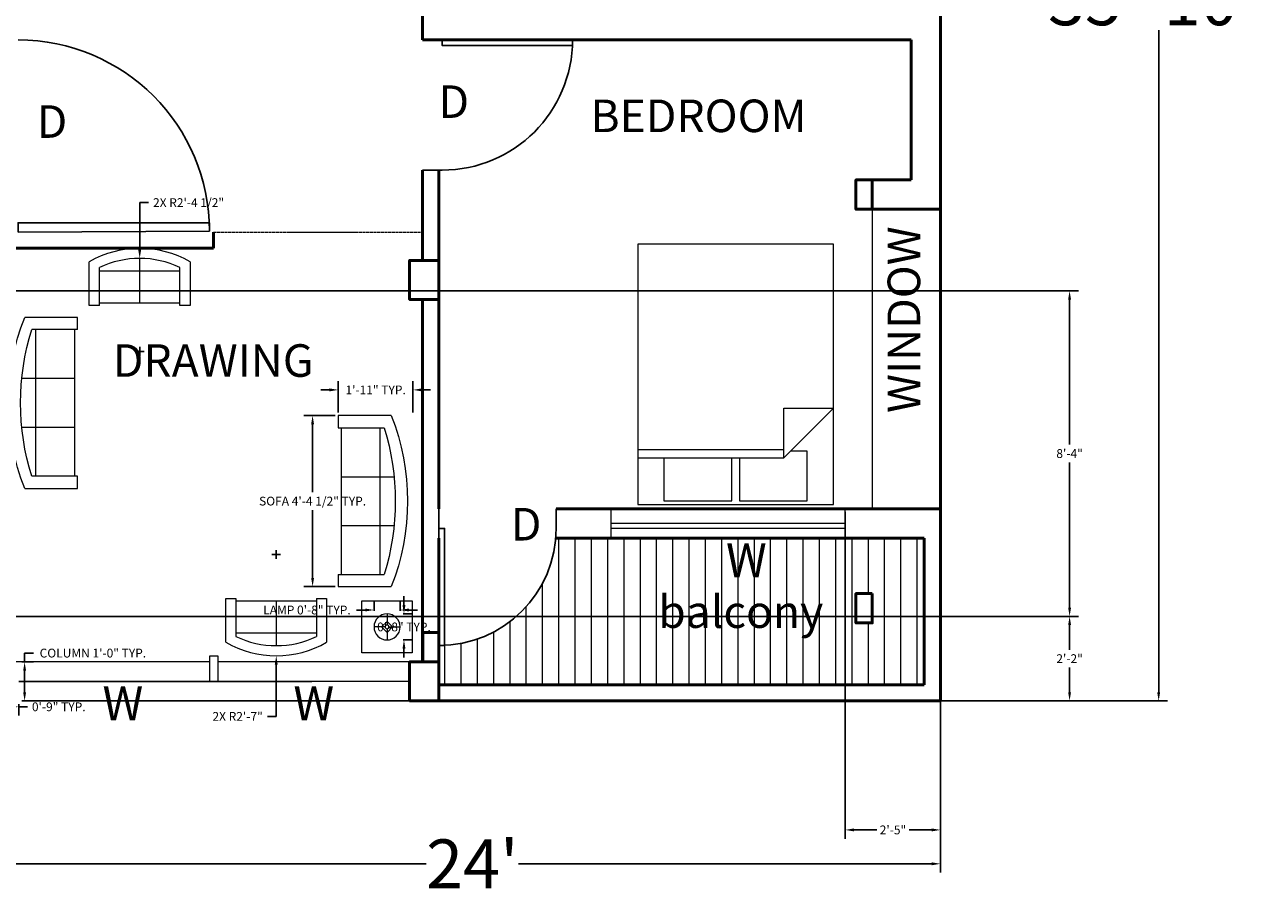
# Model space of a CAD drawing. Units: inches. Extents: x -15 to 796, y 111 to 651.
# Tile 5 of 6: x 416 to 796, y 111 to 376. Entities that reach past the tile are written whole.
import ezdxf

# ---------------------------------------------------------------- set-up
doc = ezdxf.new("R2010")
doc.units = ezdxf.units.IN
doc.header["$MEASUREMENT"] = 0
doc.linetypes.add('DASHED2', pattern=[0.375, 0.25, -0.125])
doc.layers.get('0').update_dxf_attribs({"color": 1})
for name, color, linetype, lineweight in [('A-ANNO-DIMS', 2, 'Continuous', 18), ('A-ANNO-TEXT', 7, 'Continuous', 18), ('A-AREA-IDEN', 7, 'Continuous', 25), ('A-COLS', 1, 'Continuous', 50), ('A-DOOR', 3, 'Continuous', 25), ('A-FLOR-PATT', 18, 'Continuous', 13), ('A-FURN', 8, 'Continuous', 18), ('A-GLAZ', 4, 'Continuous', 18), ('A-WALL', 7, 'Continuous', 50), ('A-WALL-OVHD', 7, 'DASHED2', 18)]:
    doc.layers.add(name, color=color, linetype=linetype, lineweight=lineweight)
doc.styles.get("Standard").update_dxf_attribs({"font": 'arial.ttf'})
doc.dimstyles.get("Standard").update_dxf_attribs({"dimscale": 15, "dimtxt": 0.18, "dimasz": 0.18, "dimexe": 0.18, "dimexo": 0.0625, "dimgap": 0.09, "dimtad": 0, "dimtih": 1, "dimtoh": 1, "dimdec": 0, "dimzin": 0, "dimdsep": 46, "dimlunit": 3, "dimtxsty": 'Standard', "dimcen": 0.09, "dimadec": 0, "dimazin": 0, "dimtfac": 1, "dimtdec": 0, "dimtofl": 0, "dimtmove": 0, "dimatfit": 3, "dimfxl": 1, "dimtolj": 1, "dimtzin": 0, "dimarcsym": 0})

# ---------------------------------------------------------------- blocks, each defined once
blk = doc.blocks.new('*U2')
for p, q in [((-36, 0), (-36, 6)), ((0, 0), (0, 6))]:
    blk.add_line(p, q)
blk.add_lwpolyline([(0, 0), (0, -36), (-1.75, -36), (-1.75, 0)], close=True)
blk.add_arc((0, 0), 36, 180, 270)
blk = doc.blocks.new('Bed - Queen')
for p, q in [((0, -80.00003), (0, 0)), ((0, 0), (59.99999, 0)), ((59.99999, 0), (59.99999, -80.00003)), ((7.99999, -1.2), (28.79998, -1.2)), ((7.99999, -14.4), (7.99999, -1.2)), ((28.79998, -1.2), (28.79998, -14.4)), ((31.19999, -1.2), (51.99999, -1.2)), ((31.19999, -14.4), (31.19999, -1.2)), ((51.99999, -1.2), (51.99999, -16.4)), ((0, -14.4), (44.8, -14.4)), ((59.99999, -29.6), (44.8, -14.4)), ((44.8, -14.4), (44.8, -29.6)), ((44.8, -16.8), (0, -16.8)), ((51.99999, -16.4), (46.79936, -16.4)), ((44.8, -29.6), (59.99999, -29.6)), ((59.99999, -80.00003), (0, -80.00003))]:
    blk.add_line(p, q)
blk = doc.blocks.new('*U4')
for p, q in [((0, 0), (0, -6)), ((-40, 0), (-40, -6))]:
    blk.add_line(p, q)
blk.add_lwpolyline([(0, 0), (0, 40), (-1.75, 40), (-1.75, 0)], close=True)
blk.add_arc((0, 0), 40, 90, 180)
blk = doc.blocks.new('Sofa - Roundback Loveseat 5 ft.')
for p, q in [((0, -32.44198), (0, -5.99998)), ((-24, -33.99998), (-24, -11.46958)), ((-23.9998, -13.38178), (23.99986, -13.38178)), ((24.00004, -33.99998), (24.00004, -11.46958)), ((-24, -32.44198), (24.00004, -32.44198))]:
    blk.add_line(p, q)
for points in [[(-24, -33.99998), (-30, -33.99998), (-30, -7.99998)], [(30.00004, -7.99998), (30.00004, -33.99998), (24.00004, -33.99998)]]:
    blk.add_lwpolyline(points)
for centre, radius, start, end in [((0, -60.24998), 60.24998, 60.13715, 119.8628), ((0, -61.38438), 55.38444, 64.32083, 115.6792)]:
    blk.add_arc(centre, radius, start, end)
blk = doc.blocks.new('Lamp - Table')
for p, q in [((0, 7), (0, 1)), ((-1, 0), (-7, 0)), ((0, 3), (-3, 0)), ((-3, 0), (0, -3)), ((3, 0), (0, 3)), ((0, -3), (3, 0)), ((1, 0), (7, 0)), ((0, -1), (0, -7))]:
    blk.add_line(p, q)
for radius in [7, 1]:
    blk.add_circle((0, 0), radius)
blk = doc.blocks.new('Sofa - Roundback 7 ft.')
for p, q in [((-36.000027, -34), (-36.000027, -11.4696)), ((-12.00002, -32.4421), (-12.00003, -6.5971)), ((11.99997, -32.4421), (11.99998, -6.5971)), ((35.99998, -34), (35.99998, -11.4696)), ((-35.999844, -13.3819), (35.9998, -13.3819)), ((-36.000027, -32.4421), (35.99998, -32.4421))]:
    blk.add_line(p, q)
for points in [[(-36.000027, -34), (-42.000027, -34), (-42.000027, -8)], [(41.99998, -8), (41.99998, -34), (35.99998, -34)]]:
    blk.add_lwpolyline(points)
for centre, radius, start, end in [((0, -114.25), 114.25, 68.43141, 111.5686), ((-0.00001, -127.1968), 121.1968, 72.72033, 107.2797)]:
    blk.add_arc(centre, radius, start, end)
blk = doc.blocks.new('*D17')
at = {"layer": 'A-ANNO-DIMS', "color": 0, "lineweight": -2, "transparency": 16777216}
for p, q in [((698.12, 598.13), (766.83, 598.13)), ((764.13, 595.43), (764.13, 392.14)), ((764.13, 170.83), (764.13, 374.11)), ((698.12, 168.13), (766.83, 168.13))]:
    blk.add_line(p, q, dxfattribs=at)
at = {"layer": 'A-ANNO-DIMS', "color": 0, "transparency": 16777216}
for points in [[(763.68, 595.43), (764.58, 595.43), (764.13, 598.13)], [(763.68, 170.83), (764.58, 170.83), (764.13, 168.13)]]:
    blk.add_solid(points, dxfattribs=at)
at = {"layer": 'Defpoints', "color": 0, "transparency": 16777216}
for p in [(697.18, 598.13), (697.18, 168.13), (764.13, 168.13)]:
    blk.add_point(p, dxfattribs=at)
at = {"layer": 'A-ANNO-DIMS', "color": 0, "transparency": 16777216, "insert": (764.13, 383.13), "char_height": 2.7, "attachment_point": 5}
blk.add_mtext('\\A1;{\\H5.55556x;35\'-10"}', dxfattribs=at)
blk = doc.blocks.new('*D18')
at = {"layer": 'A-ANNO-DIMS', "color": 0, "lineweight": -2, "transparency": 16777216}
for p, q in [((409.68, 179.19), (409.68, 115.42)), ((697.18, 179.19), (697.18, 115.42)), ((412.38, 118.12), (539.23, 118.12)), ((694.48, 118.12), (567.64, 118.12))]:
    blk.add_line(p, q, dxfattribs=at)
at = {"layer": 'A-ANNO-DIMS', "color": 0, "transparency": 16777216}
for points in [[(412.38, 118.57), (412.38, 117.67), (409.68, 118.12)], [(694.48, 118.57), (694.48, 117.67), (697.18, 118.12)]]:
    blk.add_solid(points, dxfattribs=at)
at = {"layer": 'Defpoints', "color": 0, "transparency": 16777216}
for p in [(409.68, 180.13), (697.18, 180.13), (697.18, 118.12)]:
    blk.add_point(p, dxfattribs=at)
at = {"layer": 'A-ANNO-DIMS', "color": 0, "transparency": 16777216, "insert": (553.43, 118.12), "char_height": 2.7, "attachment_point": 5}
blk.add_mtext("\\A1;{\\H5.55556x;24'}", dxfattribs=at)
blk = doc.blocks.new('DOOR-ENTRY-59IN')
blk.add_lwpolyline([(0, -0.29), (-58.71, 0), (-58.71, 2.57), (0, 2.57)], close=True)
blk.add_arc((0, 0), 58.71, 90, 180)
blk = doc.blocks.new('WIN-BEDROOM-72IN')
for p, q in [((0, 4.5), (72, 4.5)), ((0, 2.96), (72, 2.96))]:
    blk.add_line(p, q)
blk.add_lwpolyline([(0, 9), (72, 9), (72, 0), (0, 0)], close=True)
blk = doc.blocks.new('WIN-LIVING-PAIRED')
for p, q in [((62.78, 7.78), (65.45, 7.78)), ((62.78, 0), (62.78, 7.78)), ((65.45, 7.78), (65.45, 0)), ((0, 6), (62.78, 6)), ((65.45, 6), (128.5, 6)), ((4, 0), (124, 0)), ((65.45, 0), (62.78, 0))]:
    blk.add_line(p, q)
blk = doc.blocks.new('COL-9X12')
blk.add_lwpolyline([(9, 0), (0, 0), (0, 12), (9, 12)], close=True)
blk = doc.blocks.new('PIER-5X9')
blk.add_lwpolyline([(0, 9), (5, 9), (5, 0), (0, 0)], close=True)
blk = doc.blocks.new('TABLE-LAMP-STAND')
blk.add_lwpolyline([(0, 0), (15.51, 0), (15.51, 15.93), (0, 15.93)], close=True)
blk = doc.blocks.new('*D35')
at = {"layer": 'A-ANNO-DIMS', "color": 0, "lineweight": -2, "transparency": 16777216}
for p, q in [((415.98, 180.13), (415.98, 182.83)), ((415.98, 182.83), (418.68, 182.83)), ((415.12, 180.13), (418.68, 180.13)), ((415.98, 170.83), (415.98, 177.43)), ((415.12, 168.13), (418.68, 168.13))]:
    blk.add_line(p, q, dxfattribs=at)
at = {"layer": 'A-ANNO-DIMS', "color": 0, "transparency": 16777216}
for points in [[(415.53, 177.43), (416.43, 177.43), (415.98, 180.13)], [(415.53, 170.83), (416.43, 170.83), (415.98, 168.13)]]:
    blk.add_solid(points, dxfattribs=at)
at = {"layer": 'Defpoints', "color": 0, "transparency": 16777216}
for p in [(414.18, 180.13), (415.98, 180.13), (414.18, 168.13)]:
    blk.add_point(p, dxfattribs=at)
at = {"layer": 'A-ANNO-DIMS', "color": 0, "transparency": 16777216, "insert": (436.94, 182.83), "char_height": 2.7, "attachment_point": 5}
blk.add_mtext('\\A1;COLUMN 1\'-0" TYP.', dxfattribs=at)
blk = doc.blocks.new('*D36')
at = {"layer": 'A-ANNO-DIMS', "color": 0, "lineweight": -2, "transparency": 16777216}
for p, q in [((405.18, 167.19), (405.18, 163.63)), ((407.88, 166.33), (411.48, 166.33)), ((414.18, 167.19), (414.18, 163.63)), ((414.18, 166.33), (416.88, 166.33))]:
    blk.add_line(p, q, dxfattribs=at)
at = {"layer": 'A-ANNO-DIMS', "color": 0, "transparency": 16777216}
for points in [[(407.88, 166.78), (407.88, 165.88), (405.18, 166.33)], [(411.48, 166.78), (411.48, 165.88), (414.18, 166.33)]]:
    blk.add_solid(points, dxfattribs=at)
at = {"layer": 'Defpoints', "color": 0, "transparency": 16777216}
for p in [(405.18, 168.13), (414.18, 168.13), (414.18, 166.33)]:
    blk.add_point(p, dxfattribs=at)
at = {"layer": 'A-ANNO-DIMS', "color": 0, "transparency": 16777216, "insert": (426.46, 166.33), "char_height": 2.7, "attachment_point": 5}
blk.add_mtext('\\A1;0\'-9" TYP.', dxfattribs=at)
blk = doc.blocks.new('*D43')
at = {"layer": 'A-ANNO-DIMS', "color": 0, "lineweight": -2, "transparency": 16777216}
for p, q in [((511.33, 255.77), (501.69, 255.77)), ((504.39, 253.07), (504.39, 232.24)), ((504.39, 205.93), (504.39, 226.75)), ((511.33, 203.23), (501.69, 203.23))]:
    blk.add_line(p, q, dxfattribs=at)
at = {"layer": 'A-ANNO-DIMS', "color": 0, "transparency": 16777216}
for points in [[(503.94, 253.07), (504.84, 253.07), (504.39, 255.77)], [(503.94, 205.93), (504.84, 205.93), (504.39, 203.23)]]:
    blk.add_solid(points, dxfattribs=at)
at = {"layer": 'Defpoints', "color": 0, "transparency": 16777216}
for p in [(504.39, 255.77), (512.27, 255.77), (512.27, 203.23)]:
    blk.add_point(p, dxfattribs=at)
at = {"layer": 'A-ANNO-DIMS', "color": 0, "transparency": 16777216, "insert": (504.39, 229.5), "char_height": 2.7, "attachment_point": 5}
blk.add_mtext('\\A1;SOFA 4\'-4 1/2" TYP.', dxfattribs=at)
blk = doc.blocks.new('*D44')
at = {"layer": 'A-ANNO-DIMS', "color": 0, "lineweight": -2, "transparency": 16777216}
for p, q in [((512.27, 256.71), (512.27, 266.35)), ((535.21, 256.71), (535.21, 266.35)), ((509.57, 263.65), (506.87, 263.65)), ((537.91, 263.65), (540.61, 263.65))]:
    blk.add_line(p, q, dxfattribs=at)
at = {"layer": 'A-ANNO-DIMS', "color": 0, "transparency": 16777216}
for points in [[(509.57, 264.1), (509.57, 263.2), (512.27, 263.65)], [(537.91, 264.1), (537.91, 263.2), (535.21, 263.65)]]:
    blk.add_solid(points, dxfattribs=at)
at = {"layer": 'Defpoints', "color": 0, "transparency": 16777216}
for p in [(535.21, 263.65), (512.27, 255.77), (535.21, 255.77)]:
    blk.add_point(p, dxfattribs=at)
at = {"layer": 'A-ANNO-DIMS', "color": 0, "transparency": 16777216, "insert": (523.74, 263.65), "char_height": 2.7, "attachment_point": 5}
blk.add_mtext('\\A1;1\'-11" TYP.', dxfattribs=at)
blk = doc.blocks.new('*D49')
at = {"layer": 'A-ANNO-DIMS', "color": 0, "lineweight": -2, "transparency": 16777216}
for p, q in [((523.24, 195.8), (523.24, 198.76)), ((531.24, 195.8), (531.24, 198.76)), ((520.54, 196.06), (517.84, 196.06)), ((533.94, 196.06), (536.64, 196.06))]:
    blk.add_line(p, q, dxfattribs=at)
at = {"layer": 'A-ANNO-DIMS', "color": 0, "transparency": 16777216}
for points in [[(520.54, 196.51), (520.54, 195.61), (523.24, 196.06)], [(533.94, 196.51), (533.94, 195.61), (531.24, 196.06)]]:
    blk.add_solid(points, dxfattribs=at)
at = {"layer": 'Defpoints', "color": 0, "transparency": 16777216}
for p in [(523.24, 196.06), (523.24, 194.86), (531.24, 194.86)]:
    blk.add_point(p, dxfattribs=at)
at = {"layer": 'A-ANNO-DIMS', "color": 0, "transparency": 16777216, "insert": (502.66, 196.06), "char_height": 2.7, "attachment_point": 5}
blk.add_mtext('\\A1;LAMP 0\'-8" TYP.', dxfattribs=at)
blk = doc.blocks.new('*D50')
at = {"layer": 'A-ANNO-DIMS', "color": 0, "lineweight": -2, "transparency": 16777216}
for p, q in [((532.44, 197.56), (532.44, 200.26)), ((532.18, 194.86), (535.14, 194.86)), ((532.18, 186.86), (535.14, 186.86)), ((532.44, 184.16), (532.44, 181.46))]:
    blk.add_line(p, q, dxfattribs=at)
at = {"layer": 'A-ANNO-DIMS', "color": 0, "transparency": 16777216}
for points in [[(531.99, 197.56), (532.89, 197.56), (532.44, 194.86)], [(531.99, 184.16), (532.89, 184.16), (532.44, 186.86)]]:
    blk.add_solid(points, dxfattribs=at)
at = {"layer": 'Defpoints', "color": 0, "transparency": 16777216}
for p in [(531.24, 194.86), (532.44, 194.86), (531.24, 186.86)]:
    blk.add_point(p, dxfattribs=at)
at = {"layer": 'A-ANNO-DIMS', "color": 0, "transparency": 16777216, "insert": (532.44, 190.86), "char_height": 2.7, "attachment_point": 5}
blk.add_mtext('\\A1;0\'-8" TYP.', dxfattribs=at)
blk = doc.blocks.new('*D68')
at = {"layer": 'A-ANNO-DIMS', "color": 0, "lineweight": -2, "transparency": 16777216}
for p, q in [((366.85, 294.11), (739.48, 294.11)), ((736.78, 291.41), (736.78, 246.84)), ((736.78, 196.81), (736.78, 241.38)), ((366.85, 194.11), (739.48, 194.11))]:
    blk.add_line(p, q, dxfattribs=at)
at = {"layer": 'A-ANNO-DIMS', "color": 0, "transparency": 16777216}
for points in [[(736.33, 291.41), (737.23, 291.41), (736.78, 294.11)], [(736.33, 196.81), (737.23, 196.81), (736.78, 194.11)]]:
    blk.add_solid(points, dxfattribs=at)
at = {"layer": 'Defpoints', "color": 0, "transparency": 16777216}
for p in [(365.91, 294.11), (736.78, 294.11), (365.91, 194.11)]:
    blk.add_point(p, dxfattribs=at)
at = {"layer": 'A-ANNO-DIMS', "color": 0, "transparency": 16777216, "insert": (736.78, 244.11), "char_height": 2.7, "attachment_point": 5}
blk.add_mtext('\\A1;8\'-4"', dxfattribs=at)
blk = doc.blocks.new('*D77')
at = {"layer": 'A-ANNO-DIMS', "color": 0, "lineweight": -2, "transparency": 16777216}
for p, q in [((667.93, 226.19), (667.93, 125.83)), ((697.18, 226.19), (697.18, 125.83)), ((670.63, 128.53), (677.6, 128.53)), ((694.48, 128.53), (687.52, 128.53))]:
    blk.add_line(p, q, dxfattribs=at)
at = {"layer": 'A-ANNO-DIMS', "color": 0, "transparency": 16777216}
for points in [[(670.63, 128.98), (670.63, 128.08), (667.93, 128.53)], [(694.48, 128.98), (694.48, 128.08), (697.18, 128.53)]]:
    blk.add_solid(points, dxfattribs=at)
at = {"layer": 'Defpoints', "color": 0, "transparency": 16777216}
for p in [(667.93, 227.13), (697.18, 227.13), (667.93, 128.53)]:
    blk.add_point(p, dxfattribs=at)
at = {"layer": 'A-ANNO-DIMS', "color": 0, "transparency": 16777216, "insert": (682.56, 128.53), "char_height": 2.7, "attachment_point": 5}
blk.add_mtext('\\A1;2\'-5"', dxfattribs=at)
blk = doc.blocks.new('*D81')
at = {"layer": 'A-ANNO-DIMS', "color": 0, "lineweight": -2, "transparency": 16777216}
for p, q in [((410.62, 194.11), (739.48, 194.11)), ((736.78, 191.41), (736.78, 183.82)), ((736.78, 170.83), (736.78, 178.41)), ((415.12, 168.13), (739.48, 168.13))]:
    blk.add_line(p, q, dxfattribs=at)
at = {"layer": 'A-ANNO-DIMS', "color": 0, "transparency": 16777216}
for points in [[(736.33, 191.41), (737.23, 191.41), (736.78, 194.11)], [(736.33, 170.83), (737.23, 170.83), (736.78, 168.13)]]:
    blk.add_solid(points, dxfattribs=at)
at = {"layer": 'Defpoints', "color": 0, "transparency": 16777216}
for p in [(409.68, 194.11), (414.18, 168.13), (736.78, 168.13)]:
    blk.add_point(p, dxfattribs=at)
at = {"layer": 'A-ANNO-DIMS', "color": 0, "transparency": 16777216, "insert": (736.78, 181.12), "char_height": 2.7, "attachment_point": 5}
blk.add_mtext('\\A1;2\'-2"', dxfattribs=at)
blk = doc.blocks.new('*D86')
at = {"layer": 'A-ANNO-DIMS', "color": 0, "lineweight": -2, "transparency": 16777216}
for p, q in [((491.88, 213.08), (494.58, 213.08)), ((493.23, 211.73), (493.23, 214.43)), ((493.23, 163.39), (493.23, 179.32)), ((490.53, 163.39), (493.23, 163.39))]:
    blk.add_line(p, q, dxfattribs=at)
at = {"layer": 'A-ANNO-DIMS', "color": 0, "transparency": 16777216}
blk.add_solid([(492.78, 179.32), (493.68, 179.32), (493.23, 182.02)], dxfattribs=at)
at = {"layer": 'Defpoints', "color": 0, "transparency": 16777216}
for p in [(493.23, 213.08), (493.23, 182.02)]:
    blk.add_point(p, dxfattribs=at)
at = {"layer": 'A-ANNO-DIMS', "color": 0, "transparency": 16777216, "insert": (481.37, 163.39), "char_height": 2.7, "attachment_point": 5}
blk.add_mtext('\\A1;2X R2\'-7"', dxfattribs=at)
blk = doc.blocks.new('*D87')
at = {"layer": 'A-ANNO-DIMS', "color": 0, "lineweight": -2, "transparency": 16777216}
for p, q in [((454.01, 321.16), (451.31, 321.16)), ((451.31, 321.16), (451.31, 306.73)), ((449.96, 275.48), (452.66, 275.48)), ((451.31, 274.13), (451.31, 276.83))]:
    blk.add_line(p, q, dxfattribs=at)
at = {"layer": 'A-ANNO-DIMS', "color": 0, "transparency": 16777216}
blk.add_solid([(450.86, 306.73), (451.76, 306.73), (451.31, 304.03)], dxfattribs=at)
at = {"layer": 'Defpoints', "color": 0, "transparency": 16777216}
for p in [(451.31, 304.03), (451.31, 275.48)]:
    blk.add_point(p, dxfattribs=at)
at = {"layer": 'A-ANNO-DIMS', "color": 0, "transparency": 16777216, "insert": (466.31, 321.16), "char_height": 2.7, "attachment_point": 5}
blk.add_mtext('\\A1;2X R2\'-4 1/2"', dxfattribs=at)

msp = doc.modelspace()

# ---------------------------------------------------------------- hatches: boundary and pattern name
at = {"layer": 'A-FLOR-PATT'}
h = msp.add_hatch(dxfattribs=at)
h.set_pattern_fill('_USER', color=256, scale=5, angle=90, pattern_type=0)
h.set_pattern_definition([(90, (0, 0), (-5, 3e-16), [])])
h.paths.add_polyline_path([(579.06, 218.13, -0.376042), (544.93, 185.17), (544.93, 185.13), (543.18, 185.13), (543.18, 173.13), (692.18, 173.13), (692.18, 218.13)])
h.paths.add_polyline_path([(671.18, 201.09), (676.18, 201.09), (676.18, 192.09), (671.18, 192.09)], flags=16)

# ---------------------------------------------------------------- linework, layer by layer
at = {"layer": 'A-GLAZ'}
for p, q in [((676.18, 328.13), (676.18, 227.43)), ((414.18, 174.13), (504.18, 174.13))]:
    msp.add_line(p, q, dxfattribs=at)
at = {"layer": 'A-WALL'}
for p, q in [((538.18, 380.13), (538.18, 371.13)), ((697.18, 380.13), (697.18, 227.13)), ((538.18, 371.13), (688.18, 371.13)), ((676.18, 371.43), (676.18, 371.13)), ((688.18, 371.13), (688.18, 328.13)), ((538.18, 331.13), (538.18, 303.43)), ((543.18, 227.13), (543.18, 331.13)), ((688.18, 328.13), (676.18, 328.13)), ((697.18, 319.13), (676.18, 319.13)), ((473.93, 307.13), (473.93, 312.13)), ((409.68, 307.13), (473.93, 307.13)), ((538.18, 291.43), (538.18, 180.13)), ((697.18, 227.13), (579.18, 227.13)), ((697.18, 227.13), (579.18, 227.13)), ((697.18, 168.13), (697.18, 227.13)), ((543.18, 218.13), (543.18, 173.13)), ((692.18, 218.13), (579.06, 218.13)), ((692.18, 173.13), (692.18, 218.13)), ((543.18, 173.13), (692.18, 173.13)), ((534.18, 168.13), (697.18, 168.13))]:
    msp.add_line(p, q, dxfattribs=at)
at = {"layer": 'A-WALL-OVHD'}
msp.add_line((473.93, 312.13), (538.18, 312.13), dxfattribs=at)

# ---------------------------------------------------------------- block references
at = {"layer": 'A-COLS', "extrusion": (0, 0, -1), "zscale": -1}
for name, p in [('PIER-5X9', (-676.18, 319.13)), ('PIER-5X9', (-676.18, 192.09)), ('PIER-5X9', (-543.19, 180.13)), ('COL-9X12', (-543.18, 168.13))]:
    msp.add_blockref(name, p, dxfattribs=at)
at = {"layer": 'A-COLS', "extrusion": (0, 0, -1), "zscale": -1, "rotation": 180}
msp.add_blockref('COL-9X12', (-534.18, 303.43), dxfattribs=at)
at = {"layer": 'A-DOOR', "extrusion": (0, 0, -1), "zscale": -1}
msp.add_blockref('DOOR-ENTRY-59IN', (-413.99, 312.41), dxfattribs=at)
at = {"layer": 'A-DOOR', "xscale": -1, "rotation": 270}
msp.add_blockref('*U4', (544.18, 371.13), dxfattribs=at)
at = {"layer": 'A-DOOR', "xscale": -1}
msp.add_blockref('*U2', (543.18, 221.13), dxfattribs=at)
at = {"layer": 'A-FURN'}
for name, p, xscale, yscale, zscale in [('Sofa - Roundback Loveseat 5 ft.', (451.31, 307.13), 0.5154795599651856, 0.5154795599651856, 0.5154795599651856), ('Lamp - Table', (527.24, 190.86), -0.5714285204081744, 0.5714285204081744, 0.5714285204081744)]:
    msp.add_blockref(name, p, dxfattribs=dict(at, xscale=xscale, yscale=yscale, zscale=zscale))
at = {"layer": 'A-FURN', "xscale": -1, "rotation": 180}
msp.add_blockref('Bed - Queen', (604.26, 228.42), dxfattribs=at)
at = {"layer": 'A-FURN'}
for name, p, xscale, yscale, zscale, rotation in [('Sofa - Roundback 7 ft.', (411, 259.65), -0.6255113727593298, 0.6255113727593298, 0.6255113727593298, 90), ('Sofa - Roundback 7 ft.', (533.54, 229.5), -0.6255113727593298, 0.6255113727593298, 0.6255113727593298, 270), ('Sofa - Roundback Loveseat 5 ft.', (493.23, 182.02), 0.5154795599651856, 0.5154795599651856, 0.5154795599651856, 180)]:
    msp.add_blockref(name, p, dxfattribs=dict(at, xscale=xscale, yscale=yscale, zscale=zscale, rotation=rotation))
at = {"layer": 'A-FURN', "extrusion": (0, 0, -1), "zscale": -1}
msp.add_blockref('TABLE-LAMP-STAND', (-535, 182.9), dxfattribs=at)
at = {"layer": 'A-GLAZ', "extrusion": (0, 0, -1), "zscale": -1}
for name, p in [('WIN-BEDROOM-72IN', (-667.93, 218.13)), ('WIN-LIVING-PAIRED', (-538.18, 174.13))]:
    msp.add_blockref(name, p, dxfattribs=at)

# ---------------------------------------------------------------- texts
at = {"layer": 'A-ANNO-TEXT'}
msp.add_text('WINDOW', height=10, rotation=90, dxfattribs=at).set_placement((690.91, 256.56))
at = {"layer": 'A-ANNO-TEXT', "attachment_point": 3}
for s, width, gutter_width, insert, char_height in [('D', 13.2435, 1, (552.43, 357.16), 10), ('D', 13.2435, 1, (429.08, 351.05), 10), ('D', 13.2435, 1, (574.64, 227.4), 10), ('W', 19.9719, 52.27, (643.82, 216.52), 10.45), ('W', 19.9719, 52.27, (452.41, 172.64), 10.45), ('W', 19.9719, 52.27, (511.01, 172.64), 10.45)]:
    msp.add_mtext_dynamic_manual_height_columns(s, width=width, gutter_width=gutter_width, heights=[0], dxfattribs=dict(at, insert=insert, char_height=char_height))
at = {"layer": 'A-AREA-IDEN', "char_height": 10, "attachment_point": 3}
for s, width, gutter_width, insert in [('BEDROOM', 27.6124, 50, (656.06, 352.81)), ('DRAWING', 67.6028, 50, (504.66, 277.67)), ('balcony', 26.4166, 1, (661.15, 200.55))]:
    msp.add_mtext_dynamic_manual_height_columns(s, width=width, gutter_width=gutter_width, heights=[0], dxfattribs=dict(at, insert=insert))

# ---------------------------------------------------------------- dimensions: what is measured, and where the dimension line sits
at = {"layer": 'A-ANNO-DIMS'}
for base, p1, p2, angle, text, override, picture, middle in [((764.13, 168.13), (697.18, 598.13), (697.18, 168.13), 90, '{\\H5.55556x;<>}', {"dimclrd": 0, "dimclre": 0, "dimclrt": 0}, '*D17', (764.13, 383.13)), ((504.39, 255.77), (512.27, 203.23), (512.27, 255.77), 90, 'SOFA <> TYP.', {"dimdec": 1, "dimlfac": 1, "dimrnd": 0, "dimzin": 1, "dimdsep": 46, "dimlunit": 4, "dimfrac": 2}, '*D43', (504.39, 229.5)), ((523.24, 196.06), (531.24, 194.86), (523.24, 194.86), 180, 'LAMP <> TYP.', {"dimdec": 1, "dimlfac": 1, "dimrnd": 0, "dimzin": 1, "dimdsep": 46, "dimlunit": 4, "dimfrac": 2}, '*D49', (502.66, 196.06)), ((532.44, 194.86), (531.24, 186.86), (531.24, 194.86), 90, '<> TYP.', {"dimdec": 1, "dimlfac": 1, "dimrnd": 0, "dimzin": 1, "dimdsep": 46, "dimlunit": 4, "dimfrac": 2}, '*D50', (532.44, 190.86)), ((415.98, 180.13), (414.18, 168.13), (414.18, 180.13), 90, 'COLUMN <> TYP.', {"dimdec": 1, "dimlfac": 1, "dimrnd": 0, "dimzin": 1, "dimdsep": 46, "dimlunit": 4, "dimfrac": 2}, '*D35', (436.94, 182.83))]:
    dim = msp.add_linear_dim(base=base, p1=p1, p2=p2, angle=angle, text=text, dimstyle='Standard', override=override, dxfattribs=at)
    dim.commit()
    dim.dimension.update_dxf_attribs({"geometry": picture, "text_midpoint": middle})
for center, mpoint, picture, middle in [((451.311, 275.4842), (451.311, 304.0338), '*D87', (466.3111, 321.1635)), ((493.23, 213.08), (493.23, 182.02), '*D86', (481.37, 163.39))]:
    dim = msp.add_radius_dim(center=center, mpoint=mpoint, text='2X <>', dimstyle='Standard', override={"dimdec": 1, "dimlfac": 1, "dimrnd": 0, "dimzin": 1, "dimdsep": 46, "dimlunit": 4, "dimfrac": 2}, dxfattribs=at)
    dim.commit()
    dim.dimension.update_dxf_attribs({"geometry": picture, "text_midpoint": middle, "dimtype": 164})
for base, p1, p2, picture, middle in [((736.78, 294.11), (365.91, 194.11), (365.91, 294.11), '*D68', (736.78, 244.11)), ((736.78, 168.13), (409.68, 194.11), (414.18, 168.13), '*D81', (736.78, 181.12))]:
    dim = msp.add_linear_dim(base=base, p1=p1, p2=p2, angle=90, dimstyle='Standard', override={"dimdec": 1, "dimlfac": 1, "dimrnd": 0, "dimzin": 1, "dimdsep": 46, "dimlunit": 4, "dimfrac": 2}, dxfattribs=at)
    dim.commit()
    dim.dimension.update_dxf_attribs({"geometry": picture, "text_midpoint": middle})
for base, p1, p2, text, override, picture, middle in [((535.21, 263.65), (512.27, 255.77), (535.21, 255.77), '<> TYP.', {"dimdec": 1, "dimlfac": 1, "dimrnd": 0, "dimzin": 1, "dimdsep": 46, "dimlunit": 4, "dimfrac": 2}, '*D44', (523.74, 263.65)), ((697.18184818, 118.12009751), (409.68184818, 180.12661683), (697.18184818, 180.12661683), '{\\H5.55556x;<>}', {"dimclrd": 0, "dimclre": 0, "dimclrt": 0}, '*D18', (553.43184818, 118.12009751)), ((414.18, 166.33), (405.18, 168.13), (414.18, 168.13), '<> TYP.', {"dimdec": 1, "dimlfac": 1, "dimrnd": 0, "dimzin": 1, "dimdsep": 46, "dimlunit": 4, "dimfrac": 2}, '*D36', (426.46, 166.33))]:
    dim = msp.add_linear_dim(base=base, p1=p1, p2=p2, text=text, dimstyle='Standard', override=override, dxfattribs=at)
    dim.commit()
    dim.dimension.update_dxf_attribs({"geometry": picture, "text_midpoint": middle})
dim = msp.add_linear_dim(base=(667.9344, 128.5266), p1=(697.1818, 227.1266), p2=(667.9344, 227.1266), dimstyle='Standard', override={"dimdec": 1, "dimlfac": 1, "dimrnd": 0, "dimzin": 1, "dimdsep": 46, "dimlunit": 4, "dimfrac": 2}, dxfattribs=at)
dim.commit()
dim.dimension.update_dxf_attribs({"geometry": '*D77', "text_midpoint": (682.5581, 128.5266)})

doc.saveas('drawing.dxf')
